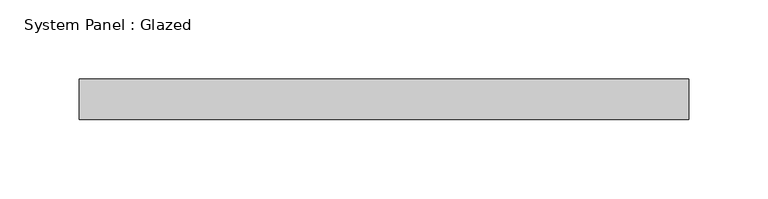
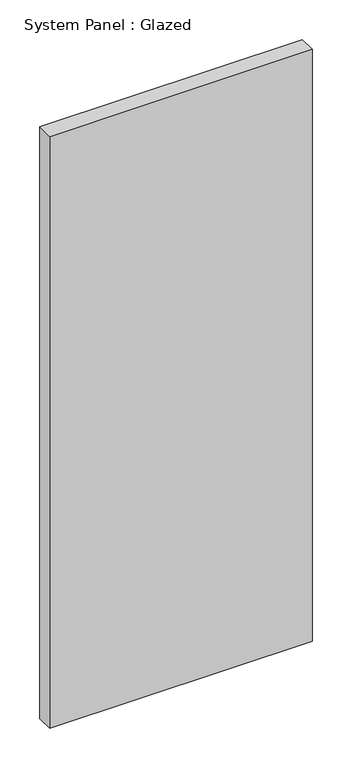
"""IFC4 building model written with IfcOpenShell, lengths in millimetres: plate geometry, System Panel : Glazed."""

from ifc_helpers import new_model, si_unit, origin, origin_with_axes, place, context, project, spatial, polyline, outline, extrude, source, transform, mapped, element, save


def system_panel_glazed_e5de8428(model_context):
    return source(origin(), model_context, "Body", "SweptSolid", [
        extrude(outline(polyline([(192.0348682, 19.05), (-192.0348682, 19.05), (-192.0348682, 44.45), (192.0348682, 44.45), (192.0348682, 19.05)])), origin_with_axes(), (0.0, 0.0, 1.0), 914.4),
    ])


if __name__ == "__main__":
    model = new_model("IFC4")
    model_context = context("Model", 3, world=origin())
    ifc_project = project(units=[si_unit("LENGTHUNIT", "METRE", prefix="MILLI")], contexts=[model_context])
    site = spatial("IfcSite", under=ifc_project)
    building = spatial("IfcBuilding", under=site)
    placement = place(None, origin())
    system_panel_glazed_shape = system_panel_glazed_e5de8428(model_context)
    element("IfcPlate", 1, ObjectType="System Panel : Glazed", at=placement, inside=building, context=model_context, shape_type="MappedRepresentation", body=[
        mapped(system_panel_glazed_shape, transform((0.0, 0.0, 0.0), x_axis=(1.0, 0.0, 0.0), y_axis=(0.0, 1.0, 0.0), z_axis=(0.0, 0.0, 1.0))),
    ])
    save(model, "model.ifc")

# Revit data of these elements
# Type "System Panel : Glazed"
#   Construction Type Id = "GSP4R"
#   Analytic Construction = "1/8 in Pilkington single glazing"
#   Visual Light Transmittance = 0.9
#   Solar Heat Gain Coefficient = 0.86
#   Heat Transfer Coefficient (U) = 1.18115 BTU/(h·ft²·°F)
# Element 1 (IfcPlate, "System Panel : Glazed")
#   Materials on its faces: "Glass"
# Materials
#   "Glass": class "Glass", colour RGB 0 128 192, transparency 0.75, Description = "Soda Lime Glass", Cost = 0
